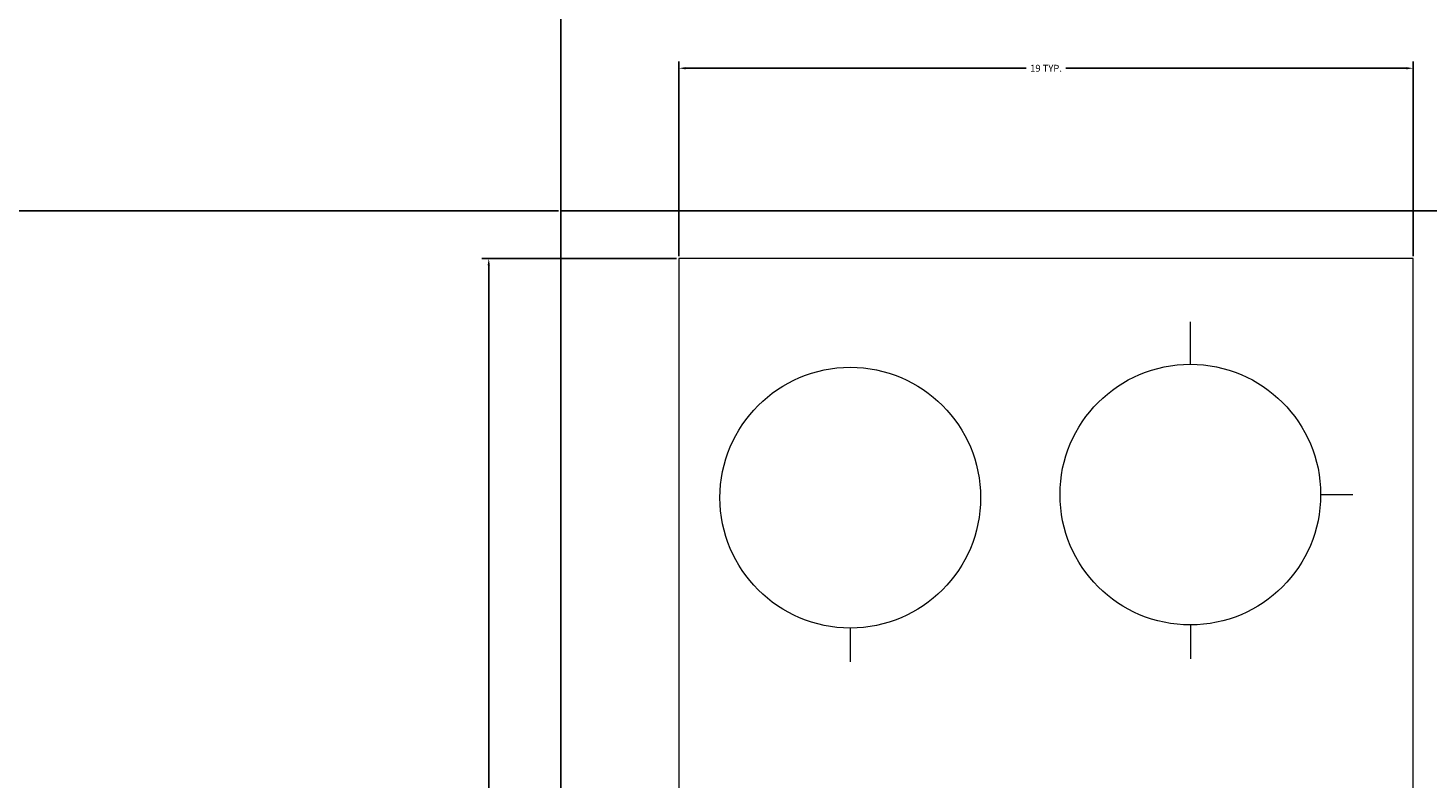
# Model space of a CAD drawing. Units: inches. Extents: x 1998 to 2588, y 1139 to 1977.
# Tile 23 of 134: x 2184 to 2220, y 1648 to 1668. Entities that reach past the tile are written whole.
import ezdxf

# ---------------------------------------------------------------- set-up
doc = ezdxf.new("R2010")
doc.units = ezdxf.units.IN
for name, color, linetype, lineweight in [('A-ANNO-DIMS', 2, 'Continuous', 18), ('A-EQPM', 21, 'Continuous', 18), ('A-FLOR-CASE', 32, 'Continuous', 25)]:
    doc.layers.add(name, color=color, linetype=linetype, lineweight=lineweight)
doc.styles.get("Standard").update_dxf_attribs({"font": 'arial.ttf'})
doc.dimstyles.get("Standard").update_dxf_attribs({"dimtxt": 0.18, "dimasz": 0.18, "dimexe": 0.18, "dimexo": 0.0625, "dimgap": 0.09, "dimtad": 0, "dimtih": 1, "dimtoh": 1, "dimdec": 4, "dimzin": 0, "dimdsep": 46, "dimtxsty": 'Standard', "dimcen": 0.09, "dimadec": 0, "dimazin": 0, "dimtfac": 1, "dimtdec": 4, "dimtofl": 0, "dimtmove": 0, "dimatfit": 3, "dimfxl": 1, "dimtolj": 1, "dimtzin": 0, "dimarcsym": 0})

# ---------------------------------------------------------------- blocks, each defined once
blk = doc.blocks.new('COOKTOP-FOUR-BURNER')
for p, q in [((13.348, 30.321), (13.348, 31.429)), ((16.748, 26.92), (17.591, 26.92)), ((4.474, 23.439), (4.474, 22.555)), ((13.348, 23.519), (13.348, 22.636)), ((4.399, 8.578), (4.399, 9.686)), ((13.348, 8.578), (13.348, 9.686)), ((0.999, 5.177), (0.172, 5.177)), ((7.8, 5.177), (8.642, 5.177)), ((9.947, 5.177), (9.12, 5.177)), ((16.748, 5.177), (17.591, 5.177)), ((4.399, 1.776), (4.399, 0.893)), ((13.348, 1.776), (13.348, 0.893))]:
    blk.add_line(p, q)
blk.add_lwpolyline([(19.165, 33.081), (0, 33.081), (0, 0), (19.165, 0)], close=True)
for centre in [(4.474, 26.84), (13.348, 26.92), (4.399, 5.177), (13.348, 5.177)]:
    blk.add_circle(centre, 3.401)
blk = doc.blocks.new('*D21')
at = {"layer": 'A-ANNO-DIMS', "color": 0, "lineweight": -2, "transparency": 16777216}
for p, q in [((2200.466, 1662.007), (2195.387, 1662.007)), ((2195.567, 1661.827), (2195.567, 1645.65)), ((2195.567, 1629.106), (2195.567, 1645.283)), ((2200.466, 1628.926), (2195.387, 1628.926))]:
    blk.add_line(p, q, dxfattribs=at)
at = {"layer": 'A-ANNO-DIMS', "color": 0, "transparency": 16777216}
for points in [[(2195.537, 1661.827), (2195.597, 1661.827), (2195.567, 1662.007)], [(2195.537, 1629.106), (2195.597, 1629.106), (2195.567, 1628.926)]]:
    blk.add_solid(points, dxfattribs=at)
at = {"layer": 'Defpoints', "color": 0, "transparency": 16777216}
for p in [(2195.567, 1662.007), (2200.529, 1662.007), (2200.529, 1628.926)]:
    blk.add_point(p, dxfattribs=at)
at = {"layer": 'A-ANNO-DIMS', "color": 0, "transparency": 16777216, "insert": (2195.567, 1645.467), "char_height": 0.18, "attachment_point": 5}
blk.add_mtext('\\A1;COOKTOP 33 TYP.', dxfattribs=at)
blk = doc.blocks.new('*D22')
at = {"layer": 'A-ANNO-DIMS', "color": 0, "lineweight": -2, "transparency": 16777216}
for p, q in [((2200.529, 1662.069), (2200.529, 1667.149)), ((2200.709, 1666.969), (2209.592, 1666.969)), ((2219.514, 1666.969), (2210.631, 1666.969)), ((2219.694, 1662.069), (2219.694, 1667.149))]:
    blk.add_line(p, q, dxfattribs=at)
at = {"layer": 'A-ANNO-DIMS', "color": 0, "transparency": 16777216}
for points in [[(2200.709, 1666.999), (2200.709, 1666.939), (2200.529, 1666.969)], [(2219.514, 1666.999), (2219.514, 1666.939), (2219.694, 1666.969)]]:
    blk.add_solid(points, dxfattribs=at)
at = {"layer": 'Defpoints', "color": 0, "transparency": 16777216}
for p in [(2219.694, 1666.969), (2200.529, 1662.007), (2219.694, 1662.007)]:
    blk.add_point(p, dxfattribs=at)
at = {"layer": 'A-ANNO-DIMS', "color": 0, "transparency": 16777216, "insert": (2210.111, 1666.969), "char_height": 0.18, "attachment_point": 5}
blk.add_mtext('\\A1;19 TYP.', dxfattribs=at)
blk = doc.blocks.new('*D36')
at = {"layer": 'A-ANNO-DIMS', "color": 0, "lineweight": -2, "transparency": 16777216}
for p, q in [((2197.45, 1663.309), (2197.45, 1977.362)), ((2222.973, 1663.309), (2222.973, 1977.362)), ((2197.63, 1977.182), (2209.746, 1977.182)), ((2222.793, 1977.182), (2210.677, 1977.182))]:
    blk.add_line(p, q, dxfattribs=at)
at = {"layer": 'A-ANNO-DIMS', "color": 0, "transparency": 16777216}
for points in [[(2197.63, 1977.212), (2197.63, 1977.152), (2197.45, 1977.182)], [(2222.793, 1977.212), (2222.793, 1977.152), (2222.973, 1977.182)]]:
    blk.add_solid(points, dxfattribs=at)
at = {"layer": 'Defpoints', "color": 0, "transparency": 16777216}
for p in [(2222.973, 1977.182), (2197.45, 1663.247), (2222.973, 1663.247)]:
    blk.add_point(p, dxfattribs=at)
at = {"layer": 'A-ANNO-DIMS', "color": 0, "transparency": 16777216, "insert": (2210.211, 1977.182), "char_height": 0.18, "attachment_point": 5}
blk.add_mtext('\\A1;25.523', dxfattribs=at)
blk = doc.blocks.new('*D37')
at = {"layer": 'A-ANNO-DIMS', "color": 0, "lineweight": -2, "transparency": 16777216}
for p, q in [((2148.455, 1612.795), (2148.455, 1977.362)), ((2197.45, 1612.795), (2197.45, 1977.362)), ((2148.635, 1977.182), (2172.73, 1977.182)), ((2197.27, 1977.182), (2173.175, 1977.182))]:
    blk.add_line(p, q, dxfattribs=at)
at = {"layer": 'A-ANNO-DIMS', "color": 0, "transparency": 16777216}
for points in [[(2148.635, 1977.212), (2148.635, 1977.152), (2148.455, 1977.182)], [(2197.27, 1977.212), (2197.27, 1977.152), (2197.45, 1977.182)]]:
    blk.add_solid(points, dxfattribs=at)
at = {"layer": 'Defpoints', "color": 0, "transparency": 16777216}
for p in [(2197.45, 1977.182), (2148.455, 1612.732), (2197.45, 1612.732)]:
    blk.add_point(p, dxfattribs=at)
at = {"layer": 'A-ANNO-DIMS', "color": 0, "transparency": 16777216, "insert": (2172.952, 1977.182), "char_height": 0.18, "attachment_point": 5}
blk.add_mtext('\\A1;49', dxfattribs=at)
blk = doc.blocks.new('*D38')
at = {"layer": 'A-ANNO-DIMS', "color": 0, "lineweight": -2, "transparency": 16777216}
for p, q in [((2197.387, 1663.247), (1997.843, 1663.247)), ((1998.023, 1663.067), (1998.023, 1638.171)), ((1998.023, 1612.912), (1998.023, 1637.808)), ((2197.387, 1612.732), (1997.843, 1612.732))]:
    blk.add_line(p, q, dxfattribs=at)
at = {"layer": 'A-ANNO-DIMS', "color": 0, "transparency": 16777216}
for points in [[(1997.993, 1663.067), (1998.053, 1663.067), (1998.023, 1663.247)], [(1997.993, 1612.912), (1998.053, 1612.912), (1998.023, 1612.732)]]:
    blk.add_solid(points, dxfattribs=at)
at = {"layer": 'Defpoints', "color": 0, "transparency": 16777216}
for p in [(1998.023, 1663.247), (2197.45, 1663.247), (2197.45, 1612.732)]:
    blk.add_point(p, dxfattribs=at)
at = {"layer": 'A-ANNO-DIMS', "color": 0, "transparency": 16777216, "insert": (1998.023, 1637.99), "char_height": 0.18, "attachment_point": 5}
blk.add_mtext('\\A1;50.51', dxfattribs=at)

msp = doc.modelspace()

# ---------------------------------------------------------------- linework, layer by layer
at = {"layer": 'A-FLOR-CASE'}
for p, q in [((2197.4499, 1612.7324), (2197.4499, 1663.2466)), ((2197.4499, 1663.2466), (2222.9729, 1663.2466))]:
    msp.add_line(p, q, dxfattribs=at)

# ---------------------------------------------------------------- block references
at = {"layer": 'A-EQPM'}
msp.add_blockref('COOKTOP-FOUR-BURNER', (2200.529, 1628.926), dxfattribs=at)

# ---------------------------------------------------------------- dimensions: what is measured, and where the dimension line sits
at = {"layer": 'A-ANNO-DIMS'}
for base, p1, p2, override, picture, middle in [((2197.4499, 1977.1824), (2148.4548, 1612.7324), (2197.4499, 1612.7324), {"dimdec": 0, "dimlfac": 1, "dimrnd": 0, "dimzin": 0, "dimdsep": 46, "dimlunit": 2}, '*D37', (2172.9524, 1977.1824)), ((2222.9729, 1977.1824), (2197.4499, 1663.2466), (2222.9729, 1663.2466), {"dimdec": 3, "dimlfac": 1, "dimrnd": 0, "dimzin": 0, "dimdsep": 46, "dimlunit": 2}, '*D36', (2210.2114, 1977.1824))]:
    dim = msp.add_linear_dim(base=base, p1=p1, p2=p2, dimstyle='Standard', override=override, dxfattribs=at)
    dim.commit()
    dim.dimension.update_dxf_attribs({"geometry": picture, "text_midpoint": middle})
dim = msp.add_linear_dim(base=(2219.6941, 1666.9688), p1=(2200.5286, 1662.0068), p2=(2219.6941, 1662.0068), text='<> TYP.', dimstyle='Standard', override={"dimdec": 0, "dimlfac": 1, "dimrnd": 0, "dimzin": 0, "dimdsep": 46, "dimlunit": 2}, dxfattribs=at)
dim.commit()
dim.dimension.update_dxf_attribs({"geometry": '*D22', "text_midpoint": (2210.1113, 1666.9688)})
dim = msp.add_linear_dim(base=(1998.0229, 1663.2466), p1=(2197.4499, 1612.7324), p2=(2197.4499, 1663.2466), angle=90, dimstyle='Standard', override={"dimdec": 2, "dimlfac": 1, "dimrnd": 0, "dimzin": 0, "dimdsep": 46, "dimlunit": 2}, dxfattribs=at)
dim.commit()
dim.dimension.update_dxf_attribs({"geometry": '*D38', "text_midpoint": (1998.0229, 1637.9895)})
dim = msp.add_linear_dim(base=(2195.5666, 1662.0068), p1=(2200.5286, 1628.9263), p2=(2200.5286, 1662.0068), angle=90, text='COOKTOP <> TYP.', dimstyle='Standard', override={"dimdec": 0, "dimlfac": 1, "dimrnd": 0, "dimzin": 0, "dimdsep": 46, "dimlunit": 2}, dxfattribs=at)
dim.commit()
dim.dimension.update_dxf_attribs({"geometry": '*D21', "text_midpoint": (2195.5666, 1645.4665)})

doc.saveas('drawing.dxf')
